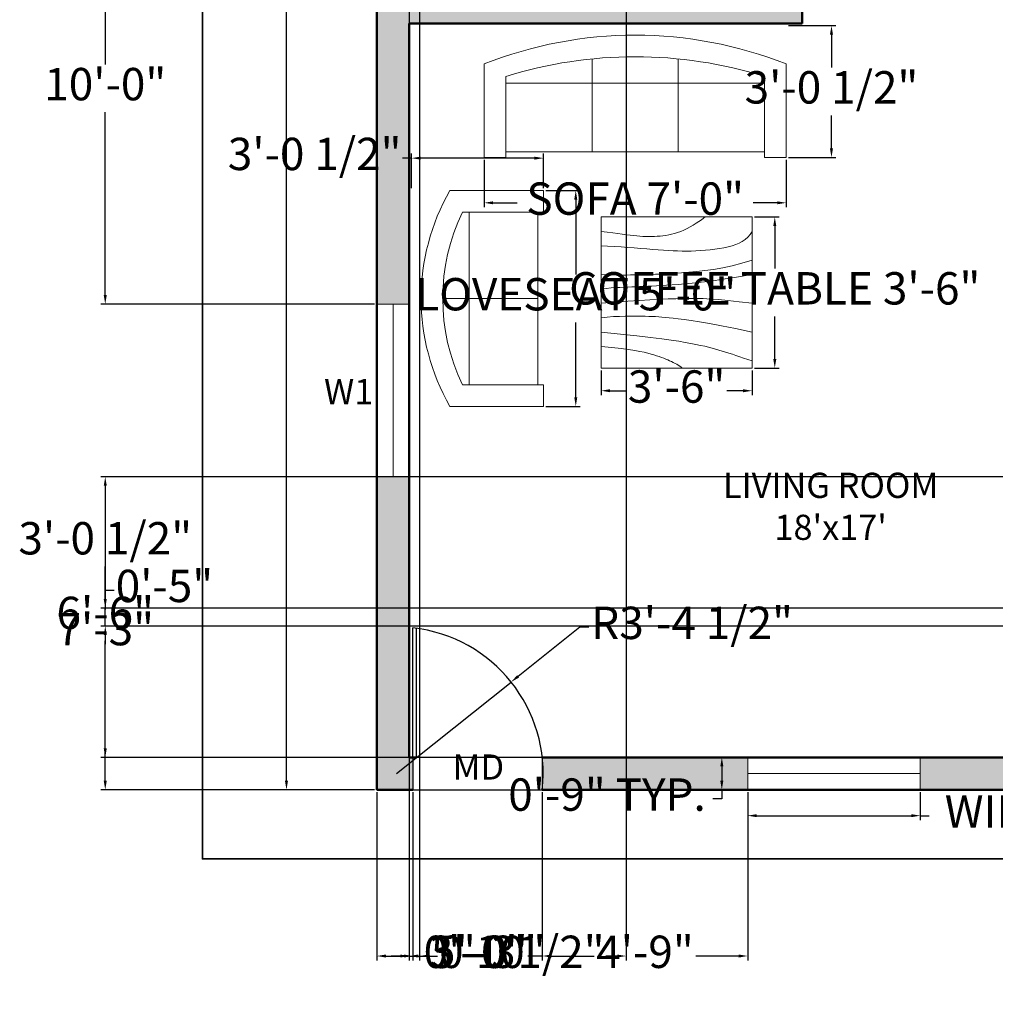
# Model space of a CAD drawing. Units: inches. Extents: x 6193 to 6719, y 6945 to 7563.
# Tile 1 of 4: x 6193 to 6464, y 6945 to 7219. Entities that reach past the tile are written whole.
import ezdxf

# ---------------------------------------------------------------- set-up
doc = ezdxf.new("R2010")
doc.units = ezdxf.units.IN
for name, color, linetype, lineweight in [('A-ANNO-DIMS', 2, 'Continuous', 18), ('A-ANNO-TEXT', 7, 'Continuous', 18), ('A-ANNO-TTLB', 7, 'Continuous', 35), ('A-AREA-IDEN', 7, 'Continuous', 25), ('A-DOOR', 3, 'Continuous', 25), ('A-FURN', 8, 'Continuous', 18), ('A-GLAZ', 4, 'Continuous', 18), ('A-WALL', 7, 'Continuous', 50)]:
    doc.layers.add(name, color=color, linetype=linetype, lineweight=lineweight)
doc.layers.add('A-WALL-PATT', color=18, linetype='Continuous', lineweight=13, true_color=0x000000)
doc.styles.get("Standard").update_dxf_attribs({"font": 'arial.ttf'})
doc.dimstyles.new('ISO-25', dxfattribs={"dimtxt": 9, "dimasz": 2.5, "dimexe": 1.25, "dimexo": 0.625, "dimgap": 2, "dimtad": 0, "dimtih": 1, "dimtoh": 1, "dimdec": 1, "dimlunit": 4, "dimtxsty": 'Standard', "dimcen": 2.5, "dimadec": 0, "dimazin": 0, "dimtfac": 0.5, "dimtdec": 1, "dimtmove": 0, "dimatfit": 3, "dimfxl": 1, "dimarcsym": 0})

# ---------------------------------------------------------------- blocks, each defined once
blk = doc.blocks.new('Sofa - Roundback 7 ft.')
for p, q in [((-12.00002, -32.4421), (-12.00003, -6.5971)), ((11.99997, -32.4421), (11.99998, -6.5971)), ((-36.000027, -34), (-36.000027, -11.4696)), ((-35.999844, -13.3819), (35.9998, -13.3819)), ((35.99998, -34), (35.99998, -11.4696)), ((-36.000027, -32.4421), (35.99998, -32.4421))]:
    blk.add_line(p, q)
for points in [[(-36.000027, -34), (-42.000027, -34), (-42.000027, -8)], [(41.99998, -8), (41.99998, -34), (35.99998, -34)]]:
    blk.add_lwpolyline(points)
for centre, radius, start, end in [((0, -114.25), 114.25, 68.43141, 111.5686), ((-0.00001, -127.1968), 121.1968, 72.72033, 107.2797)]:
    blk.add_arc(centre, radius, start, end)
blk = doc.blocks.new('Sofa - Roundback Loveseat 5 ft.')
for p, q in [((0, -32.44198), (0, -5.99998)), ((-24, -33.99998), (-24, -11.46958)), ((-23.9998, -13.38178), (23.99986, -13.38178)), ((24.00004, -33.99998), (24.00004, -11.46958)), ((-24, -32.44198), (24.00004, -32.44198))]:
    blk.add_line(p, q)
for points in [[(-24, -33.99998), (-30, -33.99998), (-30, -7.99998)], [(30.00004, -7.99998), (30.00004, -33.99998), (24.00004, -33.99998)]]:
    blk.add_lwpolyline(points)
for centre, radius, start, end in [((0, -60.24998), 60.24998, 60.13715, 119.8628), ((0, -61.38438), 55.38444, 64.32083, 115.6792)]:
    blk.add_arc(centre, radius, start, end)
blk = doc.blocks.new('Table - Square Woodgrain 42 x 42 in.')
blk.add_line((0, -42), (42, -42))
for points in [[(0, -4), (1.704, -4.2172), (3.2358, -4.4188), (4.615, -4.604), (5.8615, -4.7721), (6.9951, -4.9224), (8.0357, -5.0541), (9.0031, -5.1667), (9.9171, -5.2594), (10.7951, -5.3316), (11.6445, -5.3836), (12.4702, -5.4157), (13.277, -5.4283), (14.0698, -5.4217), (14.8535, -5.3964), (15.6331, -5.3526), (16.4133, -5.2908), (17.1986, -5.2103), (17.9913, -5.1062), (18.793, -4.9727), (19.6056, -4.8038), (20.4307, -4.5937), (21.2701, -4.3365), (22.1256, -4.0262), (22.9989, -3.6571), (23.888, -3.2272), (24.7756, -2.7516), (25.6408, -2.2491), (26.4624, -1.7387), (27.2195, -1.2395), (27.891, -0.7703), (28.456, -0.3501), (28.8934, 0.002)], [(0, -42), (0, 0), (42, 0), (42, -42)], [(0, -8), (1.8203, -8.1001), (3.6741, -8.2149), (5.5411, -8.3408), (7.4011, -8.4741), (9.2339, -8.6112), (11.0193, -8.7484), (12.7371, -8.8821), (14.3671, -9.0086), (15.8954, -9.1246), (17.3337, -9.2278), (18.6997, -9.3159), (20.0116, -9.387), (21.2871, -9.4389), (22.5442, -9.4696), (23.8008, -9.477), (25.0749, -9.459), (26.3791, -9.4137), (27.7049, -9.3403), (29.0383, -9.2382), (30.3655, -9.1068), (31.6728, -8.9455), (32.9461, -8.7535), (34.1717, -8.5304), (35.3358, -8.2756), (36.4268, -7.9863), (37.443, -7.6521), (38.3849, -7.2603), (39.253, -6.7986), (40.048, -6.2542), (40.7705, -5.6147), (41.421, -4.8674), (42, -4)], [(42, -12), (39.1784, -12.8621), (36.4519, -13.5654), (33.8246, -14.1294), (31.3004, -14.5731), (28.8832, -14.9161), (26.577, -15.1775), (24.3858, -15.3768), (22.3136, -15.5332), (20.3622, -15.6632), (18.5254, -15.7718), (16.7947, -15.8612), (15.1618, -15.9338), (13.6183, -15.9916), (12.1558, -16.0369), (10.7659, -16.0718), (9.4403, -16.0987), (8.1703, -16.1191), (6.9461, -16.1325), (5.7577, -16.1377), (4.595, -16.1335), (3.4479, -16.1188), (2.3064, -16.0924), (1.1604, -16.0532), (0, -16)], [(42, -16), (37.6529, -16.7365), (33.8802, -17.329), (30.6179, -17.7961), (27.8015, -18.1561), (25.3668, -18.4275), (23.2497, -18.6288), (21.3859, -18.7785), (19.7111, -18.8949), (18.1693, -18.9939), (16.7375, -19.0795), (15.401, -19.1534), (14.1449, -19.217), (12.9544, -19.2717), (11.8148, -19.3191), (10.7113, -19.3606), (9.6291, -19.3976), (8.5534, -19.4323), (7.47, -19.4689), (6.3643, -19.5122), (5.222, -19.5672), (4.0288, -19.6386), (2.7703, -19.7313), (1.4321, -19.8501), (0, -20)], [(0, -24), (3.9243, -23.6805), (7.4766, -23.4138), (10.6891, -23.1954), (13.5943, -23.0205), (16.2247, -22.8847), (18.6125, -22.7832), (20.7903, -22.7116), (22.7903, -22.6651), (24.6563, -22.642), (26.4764, -22.6507), (28.35, -22.7024), (30.3766, -22.8084), (32.6555, -22.98), (35.2861, -23.2283), (38.3678, -23.5645), (42, -24)], [(42, -32), (37.392, -31.017), (33.4585, -30.2231), (30.1291, -29.5949), (27.3334, -29.109), (25.0009, -28.742), (23.0612, -28.4707), (21.4439, -28.2716), (20.0786, -28.1215), (18.8998, -28.0002), (17.8609, -27.9014), (16.9206, -27.8219), (16.0371, -27.7588), (15.1691, -27.709), (14.2748, -27.6693), (13.3128, -27.6368), (12.2415, -27.6083), (11.0295, -27.5824), (9.6867, -27.5643), (8.233, -27.5608), (6.6884, -27.5787), (5.0728, -27.6248), (3.4062, -27.7058), (1.7086, -27.8286), (0, -28)], [(0, -32), (5.4026, -32.5358), (9.9494, -33.019), (13.7424, -33.4553), (16.8834, -33.8505), (19.4743, -34.2106), (21.6171, -34.5413), (23.4136, -34.8486), (24.9657, -35.1382), (26.3614, -35.4156), (27.6332, -35.6841), (28.7995, -35.9467), (29.8788, -36.2064), (30.8897, -36.4661), (31.8507, -36.7288), (32.7802, -36.9973), (33.6968, -37.2747), (34.6175, -37.5635), (35.5531, -37.8651), (36.5128, -38.1805), (37.506, -38.5108), (38.5421, -38.8568), (39.6302, -39.2197), (40.7797, -39.6004), (42, -40)], [(0, -36), (3.0098, -36.2857), (5.5354, -36.5643), (7.6368, -36.8359), (9.374, -37.1009), (10.807, -37.3597), (11.9957, -37.6126), (13.0002, -37.8599), (13.8804, -38.102), (14.6874, -38.3393), (15.4365, -38.5729), (16.1338, -38.8041), (16.7858, -39.0341), (17.3987, -39.264), (17.9787, -39.4952), (18.5322, -39.7288), (19.0655, -39.9662), (19.5832, -40.2081), (20.0842, -40.4544), (20.5657, -40.7046), (21.0249, -40.9581), (21.459, -41.2144), (21.8653, -41.4731), (22.2409, -41.7335), (22.5831, -41.9951)]]:
    blk.add_lwpolyline(points)
blk = doc.blocks.new('*D11')
at = {"layer": 'A-ANNO-DIMS', "color": 0, "lineweight": -2, "transparency": 16777216}
for p, q in [((6291.66, 7484.66), (6265.88, 7484.66)), ((6267.13, 7482.16), (6267.13, 7251.26)), ((6267.13, 7007.16), (6267.13, 7238.07)), ((6291.66, 7004.66), (6265.88, 7004.66))]:
    blk.add_line(p, q, dxfattribs=at)
at = {"layer": 'A-ANNO-DIMS', "color": 0, "transparency": 16777216}
for points in [[(6266.71, 7482.16), (6267.55, 7482.16), (6267.13, 7484.66)], [(6266.71, 7007.16), (6267.55, 7007.16), (6267.13, 7004.66)]]:
    blk.add_solid(points, dxfattribs=at)
at = {"layer": 'Defpoints', "color": 0, "transparency": 16777216}
for p in [(6292.28, 7484.66), (6267.13, 7004.66), (6292.28, 7004.66)]:
    blk.add_point(p, dxfattribs=at)
at = {"layer": 'A-ANNO-DIMS', "color": 0, "transparency": 16777216, "insert": (6267.13, 7244.66), "char_height": 9, "attachment_point": 5}
blk.add_mtext("40'", dxfattribs=at)
blk = doc.blocks.new('WIN-48IN')
for p, q in [((0, 48), (9, 48)), ((4.5, 48), (4.5, 0)), ((0, 0), (9, 0))]:
    blk.add_line(p, q)
blk = doc.blocks.new('*D14')
at = {"layer": 'A-ANNO-DIMS', "color": 0, "lineweight": -2, "transparency": 16777216}
for p, q in [((6395.41, 7004.04), (6395.41, 6996.21)), ((6443.41, 7004.04), (6443.41, 6996.21)), ((6397.91, 6997.46), (6440.91, 6997.46)), ((6443.41, 6997.46), (6445.91, 6997.46))]:
    blk.add_line(p, q, dxfattribs=at)
at = {"layer": 'A-ANNO-DIMS', "color": 0, "transparency": 16777216}
for points in [[(6397.91, 6997.88), (6397.91, 6997.05), (6395.41, 6997.46)], [(6440.91, 6997.88), (6440.91, 6997.05), (6443.41, 6997.46)]]:
    blk.add_solid(points, dxfattribs=at)
at = {"layer": 'Defpoints', "color": 0, "transparency": 16777216}
for p in [(6395.41, 7004.66), (6443.41, 7004.66), (6443.41, 6997.46)]:
    blk.add_point(p, dxfattribs=at)
at = {"layer": 'A-ANNO-DIMS', "color": 0, "transparency": 16777216, "insert": (6504.85, 6997.46), "char_height": 9, "attachment_point": 5}
blk.add_mtext('WINDOW 4\'-0" TYP.', dxfattribs=at)
blk = doc.blocks.new('*D15')
at = {"layer": 'A-ANNO-DIMS', "color": 0, "lineweight": -2, "transparency": 16777216}
for p, q in [((6394.78, 7013.66), (6386.96, 7013.66)), ((6388.21, 7011.16), (6388.21, 7007.16)), ((6394.78, 7004.66), (6386.96, 7004.66)), ((6388.21, 7004.66), (6388.21, 7002.16)), ((6388.21, 7002.16), (6385.71, 7002.16))]:
    blk.add_line(p, q, dxfattribs=at)
at = {"layer": 'A-ANNO-DIMS', "color": 0, "transparency": 16777216}
for points in [[(6387.79, 7011.16), (6388.63, 7011.16), (6388.21, 7013.66)], [(6387.79, 7007.16), (6388.63, 7007.16), (6388.21, 7004.66)]]:
    blk.add_solid(points, dxfattribs=at)
at = {"layer": 'Defpoints', "color": 0, "transparency": 16777216}
for p in [(6395.41, 7013.66), (6388.21, 7004.66), (6395.41, 7004.66)]:
    blk.add_point(p, dxfattribs=at)
at = {"layer": 'A-ANNO-DIMS', "color": 0, "transparency": 16777216, "insert": (6356.28, 7002.16), "char_height": 9, "attachment_point": 5}
blk.add_mtext('0\'-9" TYP.', dxfattribs=at)
blk = doc.blocks.new('*D24')
at = {"layer": 'A-ANNO-DIMS', "color": 0, "lineweight": -2, "transparency": 16777216}
for p, q in [((6322.11, 7179.8), (6322.11, 7166.58)), ((6406.11, 7179.8), (6406.11, 7166.58)), ((6324.61, 7167.83), (6331.3, 7167.83)), ((6403.61, 7167.83), (6396.91, 7167.83))]:
    blk.add_line(p, q, dxfattribs=at)
at = {"layer": 'A-ANNO-DIMS', "color": 0, "transparency": 16777216}
for points in [[(6324.61, 7168.24), (6324.61, 7167.41), (6322.11, 7167.83)], [(6403.61, 7168.24), (6403.61, 7167.41), (6406.11, 7167.83)]]:
    blk.add_solid(points, dxfattribs=at)
at = {"layer": 'Defpoints', "color": 0, "transparency": 16777216}
for p in [(6322.11, 7180.43), (6406.11, 7180.43), (6406.11, 7167.83)]:
    blk.add_point(p, dxfattribs=at)
at = {"layer": 'A-ANNO-DIMS', "color": 0, "transparency": 16777216, "insert": (6364.11, 7167.83), "char_height": 9, "attachment_point": 5}
blk.add_mtext('SOFA 7\'-0"', dxfattribs=at)
blk = doc.blocks.new('*D25')
at = {"layer": 'A-ANNO-DIMS', "color": 0, "lineweight": -2, "transparency": 16777216}
for p, q in [((6406.73, 7217.09), (6419.96, 7217.09)), ((6418.71, 7214.59), (6418.71, 7205.42)), ((6418.71, 7182.93), (6418.71, 7192.1)), ((6406.73, 7180.43), (6419.96, 7180.43))]:
    blk.add_line(p, q, dxfattribs=at)
at = {"layer": 'A-ANNO-DIMS', "color": 0, "transparency": 16777216}
for points in [[(6418.29, 7214.59), (6419.12, 7214.59), (6418.71, 7217.09)], [(6418.29, 7182.93), (6419.12, 7182.93), (6418.71, 7180.43)]]:
    blk.add_solid(points, dxfattribs=at)
at = {"layer": 'Defpoints', "color": 0, "transparency": 16777216}
for p in [(6406.11, 7217.09), (6418.71, 7217.09), (6406.11, 7180.43)]:
    blk.add_point(p, dxfattribs=at)
at = {"layer": 'A-ANNO-DIMS', "color": 0, "transparency": 16777216, "insert": (6418.71, 7198.76), "char_height": 9, "attachment_point": 5}
blk.add_mtext('3\'-0 1/2"', dxfattribs=at)
blk = doc.blocks.new('*D26')
at = {"layer": 'A-ANNO-DIMS', "color": 0, "lineweight": -2, "transparency": 16777216}
for p, q in [((6339.22, 7171.25), (6348.84, 7171.25)), ((6347.59, 7168.75), (6347.59, 7147.9)), ((6347.59, 7113.75), (6347.59, 7134.59)), ((6339.22, 7111.25), (6348.84, 7111.25))]:
    blk.add_line(p, q, dxfattribs=at)
at = {"layer": 'A-ANNO-DIMS', "color": 0, "transparency": 16777216}
for points in [[(6347.17, 7168.75), (6348.01, 7168.75), (6347.59, 7171.25)], [(6347.17, 7113.75), (6348.01, 7113.75), (6347.59, 7111.25)]]:
    blk.add_solid(points, dxfattribs=at)
at = {"layer": 'Defpoints', "color": 0, "transparency": 16777216}
for p in [(6338.59, 7171.25), (6347.59, 7171.25), (6338.59, 7111.25)]:
    blk.add_point(p, dxfattribs=at)
at = {"layer": 'A-ANNO-DIMS', "color": 0, "transparency": 16777216, "insert": (6347.59, 7141.25), "char_height": 9, "attachment_point": 5}
blk.add_mtext('LOVESEAT 5\'-0"', dxfattribs=at)
blk = doc.blocks.new('*D27')
at = {"layer": 'A-ANNO-DIMS', "color": 0, "lineweight": -2, "transparency": 16777216}
for p, q in [((6301.92, 7180.25), (6299.42, 7180.25)), ((6301.92, 7171.87), (6301.92, 7181.5)), ((6336.09, 7180.25), (6304.42, 7180.25)), ((6338.59, 7171.87), (6338.59, 7181.5))]:
    blk.add_line(p, q, dxfattribs=at)
at = {"layer": 'A-ANNO-DIMS', "color": 0, "transparency": 16777216}
for points in [[(6304.42, 7180.66), (6304.42, 7179.83), (6301.92, 7180.25)], [(6336.09, 7180.66), (6336.09, 7179.83), (6338.59, 7180.25)]]:
    blk.add_solid(points, dxfattribs=at)
at = {"layer": 'Defpoints', "color": 0, "transparency": 16777216}
for p in [(6301.92, 7180.25), (6301.92, 7171.25), (6338.59, 7171.25)]:
    blk.add_point(p, dxfattribs=at)
at = {"layer": 'A-ANNO-DIMS', "color": 0, "transparency": 16777216, "insert": (6274.98, 7180.25), "char_height": 9, "attachment_point": 5}
blk.add_mtext('3\'-0 1/2"', dxfattribs=at)
blk = doc.blocks.new('*D28')
at = {"layer": 'A-ANNO-DIMS', "color": 0, "lineweight": -2, "transparency": 16777216}
for p, q in [((6397.27, 7163.89), (6404.19, 7163.89)), ((6402.94, 7161.39), (6402.94, 7149.55)), ((6402.94, 7124.39), (6402.94, 7136.23)), ((6397.27, 7121.89), (6404.19, 7121.89))]:
    blk.add_line(p, q, dxfattribs=at)
at = {"layer": 'A-ANNO-DIMS', "color": 0, "transparency": 16777216}
for points in [[(6402.53, 7161.39), (6403.36, 7161.39), (6402.94, 7163.89)], [(6402.53, 7124.39), (6403.36, 7124.39), (6402.94, 7121.89)]]:
    blk.add_solid(points, dxfattribs=at)
at = {"layer": 'Defpoints', "color": 0, "transparency": 16777216}
for p in [(6396.64, 7163.89), (6402.94, 7163.89), (6396.64, 7121.89)]:
    blk.add_point(p, dxfattribs=at)
at = {"layer": 'A-ANNO-DIMS', "color": 0, "transparency": 16777216, "insert": (6402.94, 7142.89), "char_height": 9, "attachment_point": 5}
blk.add_mtext('COFFEE TABLE 3\'-6"', dxfattribs=at)
blk = doc.blocks.new('*D29')
at = {"layer": 'A-ANNO-DIMS', "color": 0, "lineweight": -2, "transparency": 16777216}
for p, q in [((6354.64, 7121.26), (6354.64, 7114.34)), ((6396.64, 7121.26), (6396.64, 7114.34)), ((6357.14, 7115.59), (6361.68, 7115.59)), ((6394.14, 7115.59), (6389.6, 7115.59))]:
    blk.add_line(p, q, dxfattribs=at)
at = {"layer": 'A-ANNO-DIMS', "color": 0, "transparency": 16777216}
for points in [[(6357.14, 7116.01), (6357.14, 7115.17), (6354.64, 7115.59)], [(6394.14, 7116.01), (6394.14, 7115.17), (6396.64, 7115.59)]]:
    blk.add_solid(points, dxfattribs=at)
at = {"layer": 'Defpoints', "color": 0, "transparency": 16777216}
for p in [(6354.64, 7121.89), (6396.64, 7121.89), (6396.64, 7115.59)]:
    blk.add_point(p, dxfattribs=at)
at = {"layer": 'A-ANNO-DIMS', "color": 0, "transparency": 16777216, "insert": (6375.64, 7115.59), "char_height": 9, "attachment_point": 5}
blk.add_mtext('3\'-6"', dxfattribs=at)
blk = doc.blocks.new('*D34')
at = {"layer": 'A-ANNO-DIMS', "color": 0, "lineweight": -2, "transparency": 16777216}
for p, q in [((6291.66, 7091.66), (6215.49, 7091.66)), ((6216.74, 7089.16), (6216.74, 7054.76)), ((6216.74, 7007.16), (6216.74, 7041.56)), ((6291.66, 7004.66), (6215.49, 7004.66))]:
    blk.add_line(p, q, dxfattribs=at)
at = {"layer": 'A-ANNO-DIMS', "color": 0, "transparency": 16777216}
for points in [[(6216.32, 7089.16), (6217.16, 7089.16), (6216.74, 7091.66)], [(6216.32, 7007.16), (6217.16, 7007.16), (6216.74, 7004.66)]]:
    blk.add_solid(points, dxfattribs=at)
at = {"layer": 'Defpoints', "color": 0, "transparency": 16777216}
for p in [(6216.74, 7091.66), (6292.28, 7091.66), (6292.28, 7004.66)]:
    blk.add_point(p, dxfattribs=at)
at = {"layer": 'A-ANNO-DIMS', "color": 0, "transparency": 16777216, "insert": (6216.74, 7048.16), "char_height": 9, "attachment_point": 5}
blk.add_mtext('7\'-3"', dxfattribs=at)
blk = doc.blocks.new('*D35')
at = {"layer": 'A-ANNO-DIMS', "color": 0, "lineweight": -2, "transparency": 16777216}
for p, q in [((6291.66, 7259.66), (6215.49, 7259.66)), ((6216.74, 7257.16), (6216.74, 7206.26)), ((6216.74, 7142.16), (6216.74, 7193.07)), ((6291.66, 7139.66), (6215.49, 7139.66))]:
    blk.add_line(p, q, dxfattribs=at)
at = {"layer": 'A-ANNO-DIMS', "color": 0, "transparency": 16777216}
for points in [[(6216.32, 7257.16), (6217.16, 7257.16), (6216.74, 7259.66)], [(6216.32, 7142.16), (6217.16, 7142.16), (6216.74, 7139.66)]]:
    blk.add_solid(points, dxfattribs=at)
at = {"layer": 'Defpoints', "color": 0, "transparency": 16777216}
for p in [(6216.74, 7259.66), (6292.28, 7259.66), (6292.28, 7139.66)]:
    blk.add_point(p, dxfattribs=at)
at = {"layer": 'A-ANNO-DIMS', "color": 0, "transparency": 16777216, "insert": (6216.74, 7199.66), "char_height": 9, "attachment_point": 5}
blk.add_mtext('10\'-0"', dxfattribs=at)
blk = doc.blocks.new('*D44')
at = {"layer": 'A-ANNO-DIMS', "color": 0, "lineweight": -2, "transparency": 16777216}
for p, q in [((6292.28, 7004.04), (6292.28, 6957.2)), ((6302.28, 7004.04), (6302.28, 6957.2)), ((6294.78, 6958.45), (6299.78, 6958.45)), ((6302.28, 6958.45), (6304.78, 6958.45))]:
    blk.add_line(p, q, dxfattribs=at)
at = {"layer": 'A-ANNO-DIMS', "color": 0, "transparency": 16777216}
for points in [[(6294.78, 6958.86), (6294.78, 6958.03), (6292.28, 6958.45)], [(6299.78, 6958.86), (6299.78, 6958.03), (6302.28, 6958.45)]]:
    blk.add_solid(points, dxfattribs=at)
at = {"layer": 'Defpoints', "color": 0, "transparency": 16777216}
for p in [(6292.28, 7004.66), (6302.28, 7004.66), (6302.28, 6958.45)]:
    blk.add_point(p, dxfattribs=at)
at = {"layer": 'A-ANNO-DIMS', "color": 0, "transparency": 16777216, "insert": (6322.24, 6958.45), "char_height": 9, "attachment_point": 5}
blk.add_mtext('0\'-10"', dxfattribs=at)
blk = doc.blocks.new('*D45')
at = {"layer": 'A-ANNO-DIMS', "color": 0, "lineweight": -2, "transparency": 16777216}
for p, q in [((6302.28, 7004.04), (6302.28, 6957.2)), ((6338.28, 7004.04), (6338.28, 6957.2)), ((6299.78, 6958.45), (6297.28, 6958.45)), ((6302.28, 6958.45), (6306.33, 6958.45)), ((6338.28, 6958.45), (6334.24, 6958.45)), ((6340.78, 6958.45), (6343.28, 6958.45))]:
    blk.add_line(p, q, dxfattribs=at)
at = {"layer": 'A-ANNO-DIMS', "color": 0, "transparency": 16777216}
for points in [[(6299.78, 6958.86), (6299.78, 6958.03), (6302.28, 6958.45)], [(6340.78, 6958.86), (6340.78, 6958.03), (6338.28, 6958.45)]]:
    blk.add_solid(points, dxfattribs=at)
at = {"layer": 'Defpoints', "color": 0, "transparency": 16777216}
for p in [(6302.28, 7004.66), (6338.28, 7004.66), (6338.28, 6958.45)]:
    blk.add_point(p, dxfattribs=at)
at = {"layer": 'A-ANNO-DIMS', "color": 0, "transparency": 16777216, "insert": (6320.28, 6958.45), "char_height": 9, "attachment_point": 5}
blk.add_mtext('3\'-0"', dxfattribs=at)
blk = doc.blocks.new('*D46')
at = {"layer": 'A-ANNO-DIMS', "color": 0, "lineweight": -2, "transparency": 16777216}
for p, q in [((6338.28, 7004.04), (6338.28, 6957.2)), ((6395.41, 7004.04), (6395.41, 6957.2)), ((6340.78, 6958.45), (6352.7, 6958.45)), ((6392.91, 6958.45), (6380.99, 6958.45))]:
    blk.add_line(p, q, dxfattribs=at)
at = {"layer": 'A-ANNO-DIMS', "color": 0, "transparency": 16777216}
for points in [[(6340.78, 6958.86), (6340.78, 6958.03), (6338.28, 6958.45)], [(6392.91, 6958.86), (6392.91, 6958.03), (6395.41, 6958.45)]]:
    blk.add_solid(points, dxfattribs=at)
at = {"layer": 'Defpoints', "color": 0, "transparency": 16777216}
for p in [(6338.28, 7004.66), (6395.41, 7004.66), (6395.41, 6958.45)]:
    blk.add_point(p, dxfattribs=at)
at = {"layer": 'A-ANNO-DIMS', "color": 0, "transparency": 16777216, "insert": (6366.85, 6958.45), "char_height": 9, "attachment_point": 5}
blk.add_mtext('4\'-9"', dxfattribs=at)
blk = doc.blocks.new('*D49')
at = {"layer": 'A-ANNO-DIMS', "color": 0, "lineweight": -2, "transparency": 16777216}
for p, q in [((6506.66, 7091.66), (6215.49, 7091.66)), ((6216.74, 7089.16), (6216.74, 7080.07)), ((6216.74, 7057.66), (6216.74, 7066.76)), ((6506.66, 7055.16), (6215.49, 7055.16))]:
    blk.add_line(p, q, dxfattribs=at)
at = {"layer": 'A-ANNO-DIMS', "color": 0, "transparency": 16777216}
for points in [[(6216.32, 7089.16), (6217.16, 7089.16), (6216.74, 7091.66)], [(6216.32, 7057.66), (6217.16, 7057.66), (6216.74, 7055.16)]]:
    blk.add_solid(points, dxfattribs=at)
at = {"layer": 'Defpoints', "color": 0, "transparency": 16777216}
for p in [(6216.74, 7091.66), (6507.28, 7091.66), (6507.28, 7055.16)]:
    blk.add_point(p, dxfattribs=at)
at = {"layer": 'A-ANNO-DIMS', "color": 0, "transparency": 16777216, "insert": (6216.74, 7073.41), "char_height": 9, "attachment_point": 5}
blk.add_mtext('3\'-0 1/2"', dxfattribs=at)
blk = doc.blocks.new('*D50')
at = {"layer": 'A-ANNO-DIMS', "color": 0, "lineweight": -2, "transparency": 16777216}
for p, q in [((6642.66, 7091.66), (6215.49, 7091.66)), ((6216.74, 7089.16), (6216.74, 7059.26)), ((6216.74, 7016.16), (6216.74, 7046.07)), ((6642.66, 7013.66), (6215.49, 7013.66))]:
    blk.add_line(p, q, dxfattribs=at)
at = {"layer": 'A-ANNO-DIMS', "color": 0, "transparency": 16777216}
for points in [[(6216.32, 7089.16), (6217.16, 7089.16), (6216.74, 7091.66)], [(6216.32, 7016.16), (6217.16, 7016.16), (6216.74, 7013.66)]]:
    blk.add_solid(points, dxfattribs=at)
at = {"layer": 'Defpoints', "color": 0, "transparency": 16777216}
for p in [(6216.74, 7091.66), (6643.28, 7091.66), (6643.28, 7013.66)]:
    blk.add_point(p, dxfattribs=at)
at = {"layer": 'A-ANNO-DIMS', "color": 0, "transparency": 16777216, "insert": (6216.74, 7052.66), "char_height": 9, "attachment_point": 5}
blk.add_mtext('6\'-6"', dxfattribs=at)
blk = doc.blocks.new('*D52')
at = {"layer": 'A-ANNO-DIMS', "color": 0, "lineweight": -2, "transparency": 16777216}
for p, q in [((6216.74, 7057.66), (6216.74, 7060.16)), ((6216.74, 7060.16), (6219.24, 7060.16)), ((6506.66, 7055.16), (6215.49, 7055.16)), ((6216.74, 7050.16), (6216.74, 7055.16)), ((6506.66, 7050.16), (6215.49, 7050.16)), ((6216.74, 7047.66), (6216.74, 7045.16))]:
    blk.add_line(p, q, dxfattribs=at)
at = {"layer": 'A-ANNO-DIMS', "color": 0, "transparency": 16777216}
for points in [[(6216.32, 7057.66), (6217.16, 7057.66), (6216.74, 7055.16)], [(6216.32, 7047.66), (6217.16, 7047.66), (6216.74, 7050.16)]]:
    blk.add_solid(points, dxfattribs=at)
at = {"layer": 'Defpoints', "color": 0, "transparency": 16777216}
for p in [(6216.74, 7055.16), (6507.28, 7055.16), (6507.28, 7050.16)]:
    blk.add_point(p, dxfattribs=at)
at = {"layer": 'A-ANNO-DIMS', "color": 0, "transparency": 16777216, "insert": (6233.2, 7060.16), "char_height": 9, "attachment_point": 5}
blk.add_mtext('0\'-5"', dxfattribs=at)
blk = doc.blocks.new('*D57')
at = {"layer": 'A-ANNO-DIMS', "color": 0, "lineweight": -2, "transparency": 16777216}
for p, q in [((6301.28, 7349.04), (6301.28, 6957.2)), ((6361.63, 7349.04), (6361.63, 6957.2)), ((6303.78, 6958.45), (6307.01, 6958.45)), ((6359.13, 6958.45), (6355.91, 6958.45))]:
    blk.add_line(p, q, dxfattribs=at)
at = {"layer": 'A-ANNO-DIMS', "color": 0, "transparency": 16777216}
for points in [[(6303.78, 6958.86), (6303.78, 6958.03), (6301.28, 6958.45)], [(6359.13, 6958.86), (6359.13, 6958.03), (6361.63, 6958.45)]]:
    blk.add_solid(points, dxfattribs=at)
at = {"layer": 'Defpoints', "color": 0, "transparency": 16777216}
for p in [(6301.28, 7349.66), (6361.63, 7349.66), (6361.63, 6958.45)]:
    blk.add_point(p, dxfattribs=at)
at = {"layer": 'A-ANNO-DIMS', "color": 0, "transparency": 16777216, "insert": (6331.46, 6958.45), "char_height": 9, "attachment_point": 5}
blk.add_mtext('5\'-0 1/2"', dxfattribs=at)
blk = doc.blocks.new('*D62')
at = {"layer": 'A-ANNO-DIMS', "color": 0, "lineweight": -2, "transparency": 16777216}
for p, q in [((6304.17, 7357.59), (6304.17, 6957.2)), ((6301.28, 7349.04), (6301.28, 6957.2)), ((6298.78, 6958.45), (6296.28, 6958.45)), ((6301.28, 6958.45), (6304.17, 6958.45)), ((6306.67, 6958.45), (6309.17, 6958.45))]:
    blk.add_line(p, q, dxfattribs=at)
at = {"layer": 'A-ANNO-DIMS', "color": 0, "transparency": 16777216}
for points in [[(6298.78, 6958.86), (6298.78, 6958.03), (6301.28, 6958.45)], [(6306.67, 6958.86), (6306.67, 6958.03), (6304.17, 6958.45)]]:
    blk.add_solid(points, dxfattribs=at)
at = {"layer": 'Defpoints', "color": 0, "transparency": 16777216}
for p in [(6304.17, 7358.21), (6301.28, 7349.66), (6304.17, 6958.45)]:
    blk.add_point(p, dxfattribs=at)
at = {"layer": 'A-ANNO-DIMS', "color": 0, "transparency": 16777216, "insert": (6323.13, 6958.45), "char_height": 9, "attachment_point": 5}
blk.add_mtext('0\'-3"', dxfattribs=at)
blk = doc.blocks.new('*D65')
at = {"layer": 'A-ANNO-DIMS', "color": 0, "lineweight": -2, "transparency": 16777216}
for p, q in [((6348.7, 7049.89), (6331.56, 7036.18)), ((6351.2, 7049.89), (6348.7, 7049.89)), ((6297.78, 7009.16), (6329.6, 7034.62))]:
    blk.add_line(p, q, dxfattribs=at)
at = {"layer": 'A-ANNO-DIMS', "color": 0, "transparency": 16777216}
blk.add_solid([(6331.3, 7036.51), (6331.82, 7035.86), (6329.6, 7034.62)], dxfattribs=at)
at = {"layer": 'Defpoints', "color": 0, "transparency": 16777216}
for p in [(6329.6, 7034.62), (6297.78, 7009.16)]:
    blk.add_point(p, dxfattribs=at)
at = {"layer": 'A-ANNO-DIMS', "color": 0, "transparency": 16777216, "insert": (6379.95, 7049.89), "char_height": 9, "attachment_point": 5}
blk.add_mtext('R3\'-4 1/2"', dxfattribs=at)

msp = doc.modelspace()

# ---------------------------------------------------------------- hatches: boundary and pattern name
at = {"layer": 'A-WALL-PATT'}
h = msp.add_hatch(color=256, dxfattribs=at)
h.dxf.hatch_style = 1
h.paths.add_polyline_path([(6529.28, 7484.66), (6292.28, 7484.66), (6292.28, 7436.66), (6301.28, 7436.66), (6301.28, 7475.66), (6469.28, 7475.66), (6469.28, 7295.66), (6475.28, 7295.66), (6479.73, 7295.66), (6479.73, 7301.66), (6475.28, 7301.66), (6475.28, 7475.66), (6529.28, 7475.66)])
h.paths.add_polyline_path([(6652.28, 7484.66), (6589.28, 7484.66), (6589.28, 7475.66), (6643.28, 7475.66), (6643.28, 7412.66), (6652.28, 7412.66)])
h.paths.add_polyline_path([(6652.28, 7364.66), (6643.28, 7364.66), (6643.28, 7301.66), (6515.73, 7301.66, -0.038405), (6515.73, 7295.66), (6565.28, 7295.66), (6565.28, 7248.66, -0.055385), (6571.28, 7248.66), (6571.28, 7295.66), (6643.28, 7295.66), (6643.28, 7271.66), (6652.28, 7271.66)])
h.paths.add_polyline_path([(6652.28, 7247.66), (6643.28, 7247.66), (6643.28, 7223.66), (6571.28, 7223.66), (6565.28, 7223.66), (6517.28, 7223.66), (6517.28, 7217.66), (6517.28, 7135.82, -0.038405), (6523.28, 7135.82), (6523.28, 7217.66), (6565.28, 7217.66), (6571.28, 7217.66), (6643.28, 7217.66), (6643.28, 7181.66), (6652.28, 7181.66)])
h.paths.add_polyline_path([(6301.28, 7217.66), (6410.54, 7217.66), (6410.54, 7223.66), (6301.28, 7223.66), (6301.28, 7259.66), (6292.28, 7259.66), (6292.28, 7139.66), (6301.28, 7139.66)])
h.paths.add_polyline_path([(6301.28, 7343.66), (6361.63, 7343.66), (6361.63, 7349.66), (6301.28, 7349.66), (6301.28, 7388.66), (6292.28, 7388.66), (6292.28, 7307.66), (6301.28, 7307.66)], flags=17)
h.paths.add_polyline_path([(6301.28, 7091.66), (6292.28, 7091.66), (6292.28, 7004.66), (6302.28, 7004.66), (6302.28, 7013.66), (6301.28, 7013.66)])
h.paths.add_polyline_path([(6395.41, 7013.66), (6338.28, 7013.66, -0.055385), (6338.28, 7004.66), (6395.41, 7004.66)])
h.paths.add_polyline_path([(6652.28, 7028.66), (6643.28, 7028.66), (6643.28, 7013.66), (6443.41, 7013.66), (6443.41, 7004.66), (6652.28, 7004.66)])
h.paths.add_polyline_path([(6652.28, 7133.66), (6643.28, 7133.66), (6643.28, 7097.66), (6523.28, 7097.66), (6517.28, 7097.66), (6517.28, 7091.66), (6523.28, 7091.66), (6643.28, 7091.66), (6643.28, 7076.66), (6652.28, 7076.66)])
h.paths.add_polyline_path([(6517.28, 7097.66), (6507.28, 7097.66), (6507.28, 7091.66), (6517.28, 7091.66)])

# ---------------------------------------------------------------- linework, layer by layer
at = {"layer": 'A-ANNO-TTLB'}
msp.add_lwpolyline([(6243.74, 7522.77), (6678.43, 7522.77), (6678.43, 6985.45), (6243.74, 6985.45)], close=True, dxfattribs=at)
at = {"layer": 'A-DOOR'}
for p, q in [((6302.28, 7013.66), (6302.28, 7049.66)), ((6303.28, 7013.66), (6303.28, 7049.54)), ((6302.28, 7013.66), (6302.28, 7004.66)), ((6338.28, 7013.66), (6338.28, 7004.66)), ((6302.28, 7004.66), (6338.28, 7004.66))]:
    msp.add_line(p, q, dxfattribs=at)
msp.add_arc((6297.78, 7009.16), 40.75, 353.6598, 83.6598, dxfattribs=at)
at = {"layer": 'A-WALL'}
for p, q in [((6292.28, 7004.66), (6292.28, 7484.66)), ((6410.54, 7223.66), (6410.54, 7217.66)), ((6301.28, 7013.66), (6301.28, 7217.66)), ((6410.54, 7217.66), (6301.28, 7217.66)), ((6303.28, 7013.66), (6301.28, 7013.66)), ((6643.28, 7013.66), (6338.28, 7013.66)), ((6302.28, 7004.66), (6292.28, 7004.66)), ((6652.28, 7004.66), (6338.28, 7004.66))]:
    msp.add_line(p, q, dxfattribs=at)

# ---------------------------------------------------------------- block references
at = {"layer": 'A-FURN'}
for name, p in [('Sofa - Roundback 7 ft.', (6364.11, 7214.43)), ('Table - Square Woodgrain 42 x 42 in.', (6354.64, 7163.89))]:
    msp.add_blockref(name, p, dxfattribs=at)
at = {"layer": 'A-FURN', "rotation": 90}
msp.add_blockref('Sofa - Roundback Loveseat 5 ft.', (6304.59, 7141.25), dxfattribs=at)
at = {"layer": 'A-GLAZ'}
msp.add_blockref('WIN-48IN', (6292.28, 7091.66), dxfattribs=at)
at = {"layer": 'A-GLAZ', "rotation": 269.9999999999992}
msp.add_blockref('WIN-48IN', (6395.41, 7013.66), dxfattribs=at)

# ---------------------------------------------------------------- texts
at = {"layer": 'A-ANNO-TEXT', "char_height": 7, "attachment_point": 1}
for s, width, insert in [('\\pxqc;W1', 21.3946, (6273.73, 7118.85)), ('\\pxqc;MD', 25.8264, (6307.6, 7014.49))]:
    msp.add_mtext_dynamic_manual_height_columns(s, width=width, gutter_width=12.5, heights=[0], dxfattribs=dict(at, insert=insert))
at = {"layer": 'A-AREA-IDEN', "insert": (6362.84, 7092.79), "char_height": 7, "attachment_point": 1}
msp.add_mtext_dynamic_manual_height_columns("\\pxqc;{\\fArial|b1|i0|c0|p34;LIVING ROOM\\P18'x17'}", width=111.2694, gutter_width=12.5, heights=[0], dxfattribs=at)

# ---------------------------------------------------------------- dimensions: what is measured, and where the dimension line sits
at = {"layer": 'A-ANNO-DIMS'}
dim = msp.add_aligned_dim(p1=(6292.28, 7484.66), p2=(6292.28, 7004.66), distance=-25.15, dimstyle='ISO-25', override={"dimclrd": 0, "dimclre": 0, "dimclrt": 0}, dxfattribs=at)
dim.commit()
dim.dimension.update_dxf_attribs({"geometry": '*D11', "text_midpoint": (6267.13, 7244.66)})
for base, p1, p2, picture, middle in [((6304.17, 6958.45), (6301.28, 7349.66), (6304.17, 7358.21), '*D62', (6323.13, 6958.45)), ((6361.6339, 6958.4457), (6301.2849, 7349.6631), (6361.6339, 7349.6631), '*D57', (6331.4594, 6958.4457)), ((6396.64, 7115.59), (6354.64, 7121.89), (6396.64, 7121.89), '*D29', (6375.64, 7115.59)), ((6302.28, 6958.45), (6292.28, 7004.66), (6302.28, 7004.66), '*D44', (6322.24, 6958.45)), ((6338.28, 6958.45), (6302.28, 7004.66), (6338.28, 7004.66), '*D45', (6320.28, 6958.45)), ((6395.41, 6958.45), (6338.28, 7004.66), (6395.41, 7004.66), '*D46', (6366.85, 6958.45))]:
    dim = msp.add_linear_dim(base=base, p1=p1, p2=p2, dimstyle='ISO-25', override={"dimdec": 1, "dimlfac": 1, "dimrnd": 0, "dimzin": 1, "dimdsep": 46, "dimlunit": 4, "dimfrac": 2}, dxfattribs=at)
    dim.commit()
    dim.dimension.update_dxf_attribs({"geometry": picture, "text_midpoint": middle})
for base, p1, p2, angle, picture, middle in [((6216.74, 7259.66), (6292.28, 7139.66), (6292.28, 7259.66), 90, '*D35', (6216.74, 7199.66)), ((6418.71, 7217.09), (6406.11, 7180.43), (6406.11, 7217.09), 90, '*D25', (6418.71, 7198.76)), ((6301.92, 7180.25), (6338.59, 7171.25), (6301.92, 7171.25), 180, '*D27', (6274.98, 7180.25)), ((6216.74, 7091.66), (6507.28, 7055.16), (6507.28, 7091.66), 90, '*D49', (6216.74, 7073.41)), ((6216.74, 7091.66), (6292.28, 7004.66), (6292.28, 7091.66), 90, '*D34', (6216.74, 7048.16)), ((6216.74, 7091.66), (6643.28, 7013.66), (6643.28, 7091.66), 90, '*D50', (6216.74, 7052.66)), ((6216.74, 7055.16), (6507.28, 7050.16), (6507.28, 7055.16), 90, '*D52', (6233.2, 7060.16))]:
    dim = msp.add_linear_dim(base=base, p1=p1, p2=p2, angle=angle, dimstyle='ISO-25', override={"dimdec": 1, "dimlfac": 1, "dimrnd": 0, "dimzin": 1, "dimdsep": 46, "dimlunit": 4, "dimfrac": 2}, dxfattribs=at)
    dim.commit()
    dim.dimension.update_dxf_attribs({"geometry": picture, "text_midpoint": middle})
for base, p1, p2, text, picture, middle in [((6406.11, 7167.83), (6322.11, 7180.43), (6406.11, 7180.43), 'SOFA <>', '*D24', (6364.11, 7167.83)), ((6443.41, 6997.46), (6395.41, 7004.66), (6443.41, 7004.66), 'WINDOW <> TYP.', '*D14', (6504.85, 6997.46))]:
    dim = msp.add_linear_dim(base=base, p1=p1, p2=p2, text=text, dimstyle='ISO-25', override={"dimdec": 1, "dimlfac": 1, "dimrnd": 0, "dimzin": 1, "dimdsep": 46, "dimlunit": 4, "dimfrac": 2}, dxfattribs=at)
    dim.commit()
    dim.dimension.update_dxf_attribs({"geometry": picture, "text_midpoint": middle})
for base, p1, p2, angle, text, picture, middle in [((6347.59, 7171.25), (6338.59, 7111.25), (6338.59, 7171.25), 90, 'LOVESEAT <>', '*D26', (6347.59, 7141.25)), ((6402.94, 7163.89), (6396.64, 7121.89), (6396.64, 7163.89), 90, 'COFFEE TABLE <>', '*D28', (6402.94, 7142.89)), ((6388.21, 7004.66), (6395.41, 7013.66), (6395.41, 7004.66), 270, '<> TYP.', '*D15', (6356.28, 7002.16))]:
    dim = msp.add_linear_dim(base=base, p1=p1, p2=p2, angle=angle, text=text, dimstyle='ISO-25', override={"dimdec": 1, "dimlfac": 1, "dimrnd": 0, "dimzin": 1, "dimdsep": 46, "dimlunit": 4, "dimfrac": 2}, dxfattribs=at)
    dim.commit()
    dim.dimension.update_dxf_attribs({"geometry": picture, "text_midpoint": middle})
dim = msp.add_radius_dim(center=(6297.7849, 7009.1631), mpoint=(6329.6048, 7034.6188), dimstyle='ISO-25', override={"dimdec": 1, "dimlfac": 1, "dimrnd": 0, "dimzin": 1, "dimdsep": 46, "dimlunit": 4, "dimfrac": 2}, dxfattribs=at)
dim.commit()
dim.dimension.update_dxf_attribs({"geometry": '*D65', "text_midpoint": (6379.9512, 7049.8922), "dimtype": 164})

doc.saveas('drawing.dxf')
